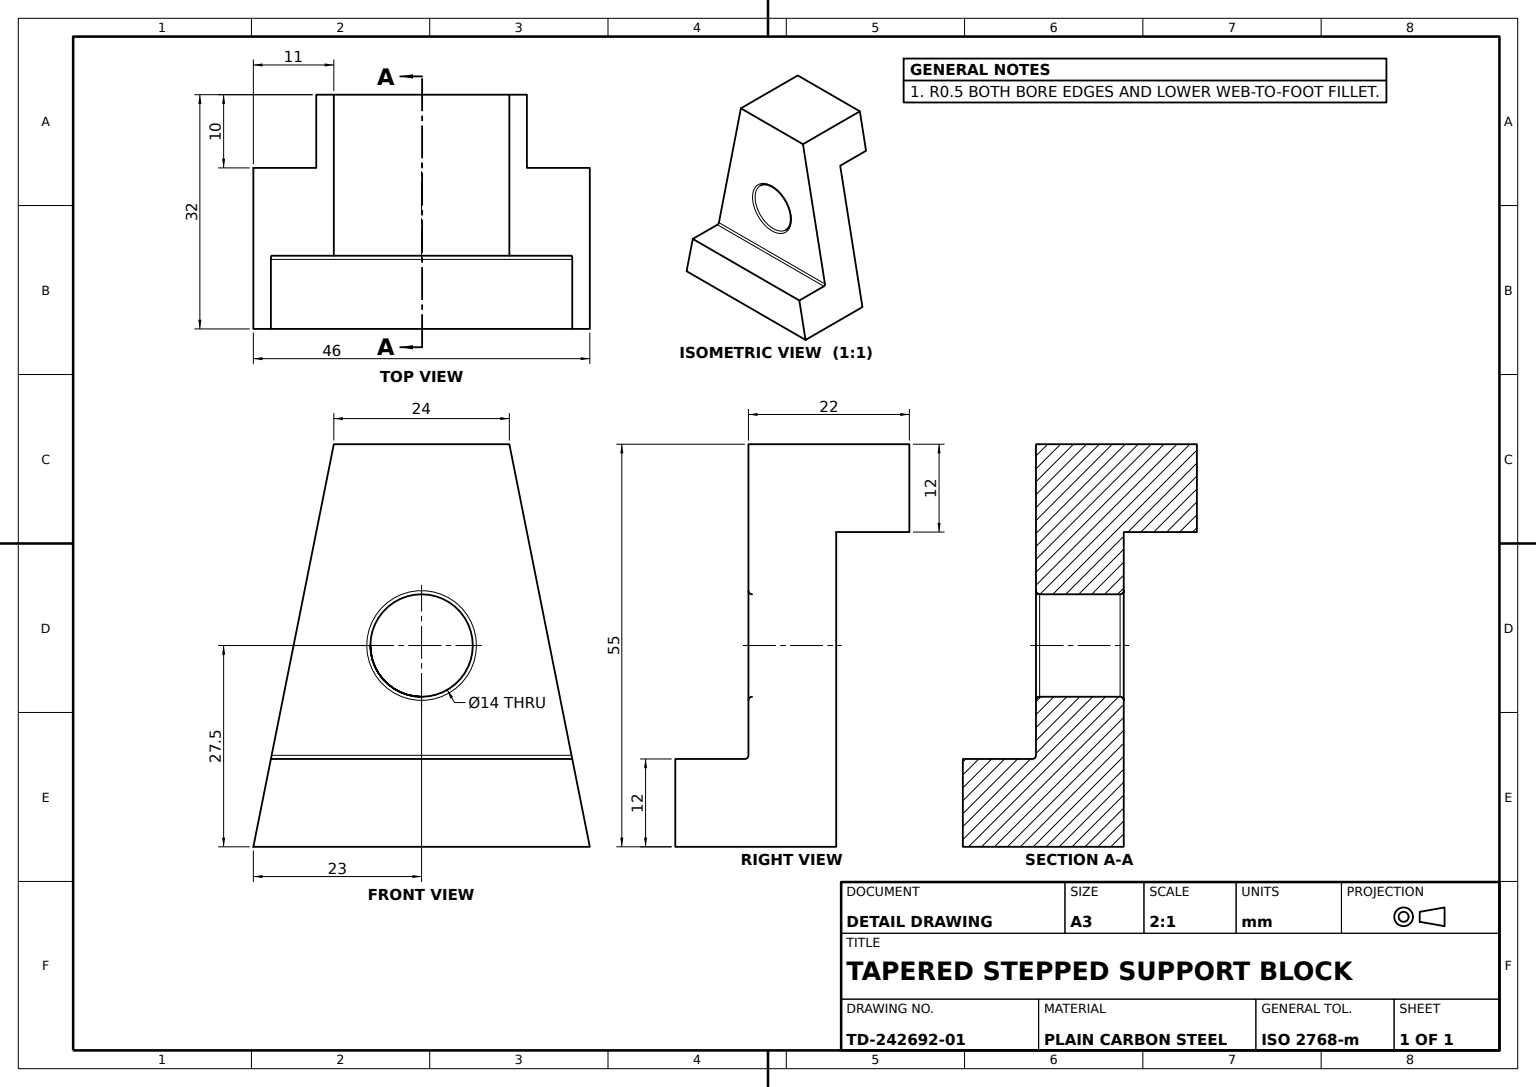
SolidWorks part; units mm, degrees
material "Plain Carbon Steel"
ref_plane "Front Plane" through (0, 0, 0) normal (0, 0, 1) x (1, 0, 0)
ref_plane "Top Plane" through (0, 0, 0) normal (0, 1, 0) x (1, 0, 0)
ref_plane "Right Plane" through (0, 0, 0) normal (1, 0, 0) x (0, 0, -1)
sketch "Bracket Profile Sketch" plane through (0, 0, 0) normal (0, 0, 1) x (1, 0, 0)
  line L0 (0, 0) -> (22, 0)
  line L1 (22, 0) -> (22, 12)
  line L2 (22, 12) -> (12, 12)
  line L3 (12, 12) -> (12, 55)
  line L4 (12, 55) -> (-10, 55)
  line L5 (-10, 55) -> (-10, 43)
  line L6 (-10, 43) -> (0, 43)
  line L7 (0, 43) -> (0, 0)
  dimension "D1" = 12
  dimension "D2" = 32
  dimension "D3" = 12
  dimension "D4" = 55
  dimension "D5" = 12
  dimension "D6" = 22
  dimension "D7" = 10
extrude "Bracket Body" add sketch "Bracket Profile Sketch" along normal blind 46
sketch "Taper Cut Sketch" plane through (22, 0, 0) normal (1, 0, 0) x (0, 0, -1)
  line L0 (-46, 0) -> (-35, 55)
  line L1 (-46, 55) -> (0, 55) construction
  line L2 (-35, 55) -> (-46, 55)
  line L3 (-46, 55) -> (-46, 0)
  line L4 (0, 0) -> (0, 55)
  line L5 (0, 55) -> (-11, 55)
  line L6 (-11, 55) -> (0, 0)
  dimension "D1" = 24
  dimension "D2" = 11
extrude "Tapered Side Cut" cut sketch "Taper Cut Sketch" against normal blind 46
sketch "Bore Sketch" plane through (0, 0, 0) normal (-1, 0, 0) x (0, 0, 1)
  line L0 (23, 55) -> (23, 0) construction
  line L1 (35, 55) -> (11, 55) construction
  line L2 (46, 0) -> (0, 0) construction
  circle A0 centre (23, 27.5) radius 7
  dimension "D1" = 14
extrude "Through Bore Ø14" cut sketch "Bore Sketch" against normal blind 46
fillet "Bore Edge Fillet R0.5 A" radius 0.5 1 edges at (12, 27.5, 30)
fillet "Bore Edge Fillet R0.5 B" radius 0.5 1 edges at (0, 20.5, 23)
fillet "Step Edge Fillet R0.5" radius 0.5 1 edges at (12, 12, 23)
